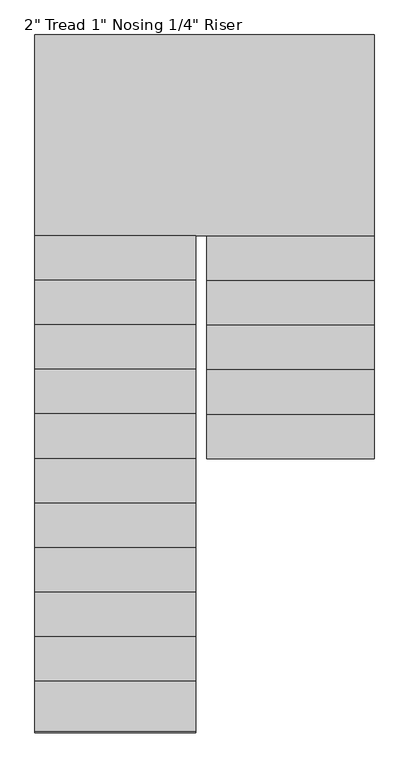
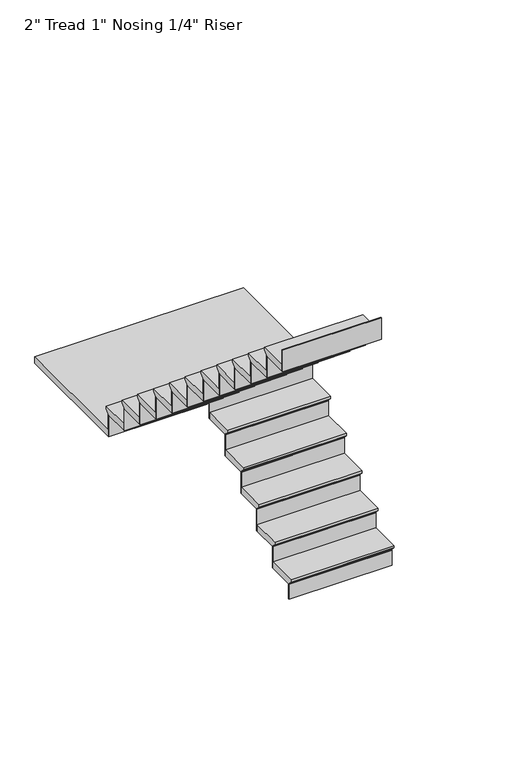
"""IFC4 building model written with IfcOpenShell, lengths in millimetres: stair flight geometry."""

from ifc_helpers import new_model, si_unit, origin, place, context, project, spatial, faceted_brep, source, transform, mapped, element, save


def stair_flight_16fb6ac5(model_context):
    return source(origin(), model_context, "Body", "Brep", [
        faceted_brep([(-3749.597125, 2714.6319226, 36573.8833333), (-3749.597125, 2714.6319226, 36592.9333333), (-4512.2136682, 2714.6319226, 36592.9333333), (-4512.2136682, 2714.6319226, 36573.8833333), (-3749.597125, 2740.0319226, 36548.4833333), (-4512.2136682, 2740.0319226, 36548.4833333), (-3749.597125, 2943.2319226, 36592.9333333), (-4512.2136682, 2943.2319226, 36592.9333333), (-4512.2136682, 2740.0319226, 36542.1333333), (-4512.2136682, 2943.2319226, 36542.1333333), (-3749.597125, 2943.2319226, 36542.1333333), (-3749.597125, 2740.0319226, 36542.1333333)], [[[0, 1, 2, 3]], [[4, 0, 3, 5]], [[2, 1, 6, 7]], [[8, 9, 10, 11]], [[2, 7, 9, 8, 5, 3]], [[8, 11, 4, 5]], [[6, 1, 0, 4, 11, 10]], [[7, 6, 10, 9]]]),
        faceted_brep([(-3749.597125, 2740.0319226, 36542.1333333), (-3749.597125, 2740.0319226, 36423.6), (-3749.597125, 2746.3819226, 36423.6), (-3749.597125, 2746.3819226, 36542.1333333), (-4512.2136682, 2740.0319226, 36542.1333333), (-4512.2136682, 2746.3819226, 36542.1333333), (-4512.2136682, 2746.3819226, 36423.6), (-4512.2136682, 2740.0319226, 36423.6)], [[[0, 1, 2, 3]], [[4, 5, 6, 7]], [[1, 0, 4, 7]], [[2, 1, 7, 6]], [[3, 2, 6, 5]], [[0, 3, 5, 4]]]),
        faceted_brep([(-3749.597125, 2943.2319226, 36711.4666667), (-3749.597125, 2943.2319226, 36542.1333333), (-3749.597125, 2949.5819226, 36542.1333333), (-3749.597125, 2949.5819226, 36711.4666667), (-4512.2136682, 2943.2319226, 36711.4666667), (-4512.2136682, 2949.5819226, 36711.4666667), (-4512.2136682, 2949.5819226, 36542.1333333), (-4512.2136682, 2943.2319226, 36542.1333333)], [[[0, 1, 2, 3]], [[4, 5, 6, 7]], [[1, 0, 4, 7]], [[2, 1, 7, 6]], [[3, 2, 6, 5]], [[0, 3, 5, 4]]]),
        faceted_brep([(-4512.2136682, 2917.8319226, 36762.2666667), (-3749.597125, 2917.8319226, 36762.2666667), (-3749.597125, 3146.4319226, 36762.2666667), (-4512.2136682, 3146.4319226, 36762.2666667), (-4512.2136682, 2943.2319226, 36711.4666667), (-4512.2136682, 3146.4319226, 36711.4666667), (-3749.597125, 3146.4319226, 36711.4666667), (-3749.597125, 2943.2319226, 36711.4666667), (-4512.2136682, 2943.2319226, 36717.8166667), (-4512.2136682, 2917.8319226, 36743.2166667), (-3749.597125, 2943.2319226, 36717.8166667), (-3749.597125, 2917.8319226, 36743.2166667)], [[[0, 1, 2, 3]], [[4, 5, 6, 7]], [[0, 3, 5, 4, 8, 9]], [[4, 7, 10, 8]], [[2, 1, 11, 10, 7, 6]], [[3, 2, 6, 5]], [[11, 1, 0, 9]], [[10, 11, 9, 8]]]),
        faceted_brep([(-3749.597125, 3146.4319226, 36880.8), (-3749.597125, 3146.4319226, 36711.4666667), (-3749.597125, 3152.7819226, 36711.4666667), (-3749.597125, 3152.7819226, 36880.8), (-4512.2136682, 3146.4319226, 36880.8), (-4512.2136682, 3152.7819226, 36880.8), (-4512.2136682, 3152.7819226, 36711.4666667), (-4512.2136682, 3146.4319226, 36711.4666667)], [[[0, 1, 2, 3]], [[4, 5, 6, 7]], [[1, 0, 4, 7]], [[2, 1, 7, 6]], [[3, 2, 6, 5]], [[0, 3, 5, 4]]]),
        faceted_brep([(-4512.2136682, 3121.0319226, 36931.6), (-3749.597125, 3121.0319226, 36931.6), (-3749.597125, 3349.6319226, 36931.6), (-4512.2136682, 3349.6319226, 36931.6), (-4512.2136682, 3146.4319226, 36880.8), (-4512.2136682, 3349.6319226, 36880.8), (-3749.597125, 3349.6319226, 36880.8), (-3749.597125, 3146.4319226, 36880.8), (-4512.2136682, 3146.4319226, 36887.15), (-4512.2136682, 3121.0319226, 36912.55), (-3749.597125, 3146.4319226, 36887.15), (-3749.597125, 3121.0319226, 36912.55)], [[[0, 1, 2, 3]], [[4, 5, 6, 7]], [[0, 3, 5, 4, 8, 9]], [[4, 7, 10, 8]], [[2, 1, 11, 10, 7, 6]], [[3, 2, 6, 5]], [[11, 1, 0, 9]], [[10, 11, 9, 8]]]),
        faceted_brep([(-3749.597125, 3349.6319226, 37050.1333333), (-3749.597125, 3349.6319226, 36880.8), (-3749.597125, 3355.9819226, 36880.8), (-3749.597125, 3355.9819226, 37050.1333333), (-4512.2136682, 3349.6319226, 37050.1333333), (-4512.2136682, 3355.9819226, 37050.1333333), (-4512.2136682, 3355.9819226, 36880.8), (-4512.2136682, 3349.6319226, 36880.8)], [[[0, 1, 2, 3]], [[4, 5, 6, 7]], [[1, 0, 4, 7]], [[2, 1, 7, 6]], [[3, 2, 6, 5]], [[0, 3, 5, 4]]]),
        faceted_brep([(-4512.2136682, 3324.2319226, 37100.9333333), (-3749.597125, 3324.2319226, 37100.9333333), (-3749.597125, 3552.8319226, 37100.9333333), (-4512.2136682, 3552.8319226, 37100.9333333), (-4512.2136682, 3349.6319226, 37050.1333333), (-4512.2136682, 3552.8319226, 37050.1333333), (-3749.597125, 3552.8319226, 37050.1333333), (-3749.597125, 3349.6319226, 37050.1333333), (-4512.2136682, 3349.6319226, 37056.4833333), (-4512.2136682, 3324.2319226, 37081.8833333), (-3749.597125, 3349.6319226, 37056.4833333), (-3749.597125, 3324.2319226, 37081.8833333)], [[[0, 1, 2, 3]], [[4, 5, 6, 7]], [[0, 3, 5, 4, 8, 9]], [[4, 7, 10, 8]], [[2, 1, 11, 10, 7, 6]], [[3, 2, 6, 5]], [[11, 1, 0, 9]], [[10, 11, 9, 8]]]),
        faceted_brep([(-3749.597125, 3552.8319226, 37219.4666667), (-3749.597125, 3552.8319226, 37050.1333333), (-3749.597125, 3559.1819226, 37050.1333333), (-3749.597125, 3559.1819226, 37219.4666667), (-4512.2136682, 3552.8319226, 37219.4666667), (-4512.2136682, 3559.1819226, 37219.4666667), (-4512.2136682, 3559.1819226, 37050.1333333), (-4512.2136682, 3552.8319226, 37050.1333333)], [[[0, 1, 2, 3]], [[4, 5, 6, 7]], [[1, 0, 4, 7]], [[2, 1, 7, 6]], [[3, 2, 6, 5]], [[0, 3, 5, 4]]]),
        faceted_brep([(-4512.2136682, 3527.4319226, 37270.2666667), (-3749.597125, 3527.4319226, 37270.2666667), (-3749.597125, 3756.0319226, 37270.2666667), (-4512.2136682, 3756.0319226, 37270.2666667), (-4512.2136682, 3552.8319226, 37219.4666667), (-4512.2136682, 3756.0319226, 37219.4666667), (-3749.597125, 3756.0319226, 37219.4666667), (-3749.597125, 3552.8319226, 37219.4666667), (-4512.2136682, 3552.8319226, 37225.8166667), (-4512.2136682, 3527.4319226, 37251.2166667), (-3749.597125, 3552.8319226, 37225.8166667), (-3749.597125, 3527.4319226, 37251.2166667)], [[[0, 1, 2, 3]], [[4, 5, 6, 7]], [[0, 3, 5, 4, 8, 9]], [[4, 7, 10, 8]], [[2, 1, 11, 10, 7, 6]], [[3, 2, 6, 5]], [[11, 1, 0, 9]], [[10, 11, 9, 8]]]),
        faceted_brep([(-3749.597125, 3756.0319226, 37388.8), (-3749.597125, 3756.0319226, 37219.4666667), (-3749.597125, 3762.3819226, 37219.4666667), (-3749.597125, 3762.3819226, 37388.8), (-4512.2136682, 3756.0319226, 37388.8), (-4512.2136682, 3762.3819226, 37388.8), (-4512.2136682, 3762.3819226, 37219.4666667), (-4512.2136682, 3756.0319226, 37219.4666667)], [[[0, 1, 2, 3]], [[4, 5, 6, 7]], [[1, 0, 4, 7]], [[2, 1, 7, 6]], [[3, 2, 6, 5]], [[0, 3, 5, 4]]]),
        faceted_brep([(-4563.0136682, 3705.2319226, 37439.6), (-4563.0136682, 3730.6319226, 37439.6), (-3749.597125, 3730.6319226, 37439.6), (-3749.597125, 4645.0319226, 37439.6), (-5295.0246464, 4645.0319226, 37439.6), (-5295.0246464, 3705.2319226, 37439.6), (-4563.0136682, 3730.6319226, 37388.8), (-4563.0136682, 3705.2319226, 37388.8), (-5295.0246464, 3705.2319226, 37388.8), (-5295.0246464, 4645.0319226, 37388.8), (-3749.597125, 4645.0319226, 37388.8), (-3749.597125, 3756.0319226, 37388.8), (-4512.2136682, 3756.0319226, 37388.8), (-4512.2136682, 3730.6319226, 37388.8), (-4512.2136682, 3730.6319226, 37420.55), (-3749.597125, 3730.6319226, 37420.55), (-4512.2136682, 3756.0319226, 37395.15), (-3749.597125, 3756.0319226, 37395.15)], [[[0, 1, 2, 3, 4, 5]], [[6, 7, 8, 9, 10, 11, 12, 13]], [[1, 0, 7, 6]], [[2, 1, 6, 13, 14, 15]], [[13, 12, 16, 14]], [[12, 11, 17, 16]], [[3, 2, 15, 17, 11, 10]], [[4, 3, 10, 9]], [[5, 4, 9, 8]], [[0, 5, 8, 7]], [[17, 15, 14, 16]]]),
        faceted_brep([(-5295.0246464, 3705.2319226, 37558.1333333), (-5295.0246464, 3705.2319226, 37388.8), (-5295.0246464, 3698.8819226, 37388.8), (-5295.0246464, 3698.8819226, 37558.1333333), (-4563.0136682, 3705.2319226, 37558.1333333), (-4563.0136682, 3698.8819226, 37558.1333333), (-4563.0136682, 3698.8819226, 37388.8), (-4563.0136682, 3705.2319226, 37388.8)], [[[0, 1, 2, 3]], [[4, 5, 6, 7]], [[1, 0, 4, 7]], [[2, 1, 7, 6]], [[3, 2, 6, 5]], [[0, 3, 5, 4]]]),
        faceted_brep([(-4563.0136682, 3730.6319226, 37608.9333333), (-5295.0246464, 3730.6319226, 37608.9333333), (-5295.0246464, 3502.0319226, 37608.9333333), (-4563.0136682, 3502.0319226, 37608.9333333), (-4563.0136682, 3705.2319226, 37558.1333333), (-4563.0136682, 3502.0319226, 37558.1333333), (-5295.0246464, 3502.0319226, 37558.1333333), (-5295.0246464, 3705.2319226, 37558.1333333), (-4563.0136682, 3705.2319226, 37564.4833333), (-4563.0136682, 3730.6319226, 37589.8833333), (-5295.0246464, 3705.2319226, 37564.4833333), (-5295.0246464, 3730.6319226, 37589.8833333)], [[[0, 1, 2, 3]], [[4, 5, 6, 7]], [[0, 3, 5, 4, 8, 9]], [[4, 7, 10, 8]], [[2, 1, 11, 10, 7, 6]], [[3, 2, 6, 5]], [[11, 1, 0, 9]], [[10, 11, 9, 8]]]),
        faceted_brep([(-5295.0246464, 3502.0319226, 37727.4666667), (-5295.0246464, 3502.0319226, 37558.1333333), (-5295.0246464, 3495.6819226, 37558.1333333), (-5295.0246464, 3495.6819226, 37727.4666667), (-4563.0136682, 3502.0319226, 37727.4666667), (-4563.0136682, 3495.6819226, 37727.4666667), (-4563.0136682, 3495.6819226, 37558.1333333), (-4563.0136682, 3502.0319226, 37558.1333333)], [[[0, 1, 2, 3]], [[4, 5, 6, 7]], [[1, 0, 4, 7]], [[2, 1, 7, 6]], [[3, 2, 6, 5]], [[0, 3, 5, 4]]]),
        faceted_brep([(-4563.0136682, 3527.4319226, 37778.2666667), (-5295.0246464, 3527.4319226, 37778.2666667), (-5295.0246464, 3298.8319226, 37778.2666667), (-4563.0136682, 3298.8319226, 37778.2666667), (-4563.0136682, 3502.0319226, 37727.4666667), (-4563.0136682, 3298.8319226, 37727.4666667), (-5295.0246464, 3298.8319226, 37727.4666667), (-5295.0246464, 3502.0319226, 37727.4666667), (-4563.0136682, 3502.0319226, 37733.8166667), (-4563.0136682, 3527.4319226, 37759.2166667), (-5295.0246464, 3502.0319226, 37733.8166667), (-5295.0246464, 3527.4319226, 37759.2166667)], [[[0, 1, 2, 3]], [[4, 5, 6, 7]], [[0, 3, 5, 4, 8, 9]], [[4, 7, 10, 8]], [[2, 1, 11, 10, 7, 6]], [[3, 2, 6, 5]], [[11, 1, 0, 9]], [[10, 11, 9, 8]]]),
        faceted_brep([(-5295.0246464, 3298.8319226, 37896.8), (-5295.0246464, 3298.8319226, 37727.4666667), (-5295.0246464, 3292.4819226, 37727.4666667), (-5295.0246464, 3292.4819226, 37896.8), (-4563.0136682, 3298.8319226, 37896.8), (-4563.0136682, 3292.4819226, 37896.8), (-4563.0136682, 3292.4819226, 37727.4666667), (-4563.0136682, 3298.8319226, 37727.4666667)], [[[0, 1, 2, 3]], [[4, 5, 6, 7]], [[1, 0, 4, 7]], [[2, 1, 7, 6]], [[3, 2, 6, 5]], [[0, 3, 5, 4]]]),
        faceted_brep([(-4563.0136682, 3324.2319226, 37947.6), (-5295.0246464, 3324.2319226, 37947.6), (-5295.0246464, 3095.6319226, 37947.6), (-4563.0136682, 3095.6319226, 37947.6), (-4563.0136682, 3298.8319226, 37896.8), (-4563.0136682, 3095.6319226, 37896.8), (-5295.0246464, 3095.6319226, 37896.8), (-5295.0246464, 3298.8319226, 37896.8), (-4563.0136682, 3298.8319226, 37903.15), (-4563.0136682, 3324.2319226, 37928.55), (-5295.0246464, 3298.8319226, 37903.15), (-5295.0246464, 3324.2319226, 37928.55)], [[[0, 1, 2, 3]], [[4, 5, 6, 7]], [[0, 3, 5, 4, 8, 9]], [[4, 7, 10, 8]], [[2, 1, 11, 10, 7, 6]], [[3, 2, 6, 5]], [[11, 1, 0, 9]], [[10, 11, 9, 8]]]),
        faceted_brep([(-5295.0246464, 3095.6319226, 38066.1333333), (-5295.0246464, 3095.6319226, 37896.8), (-5295.0246464, 3089.2819226, 37896.8), (-5295.0246464, 3089.2819226, 38066.1333333), (-4563.0136682, 3095.6319226, 38066.1333333), (-4563.0136682, 3089.2819226, 38066.1333333), (-4563.0136682, 3089.2819226, 37896.8), (-4563.0136682, 3095.6319226, 37896.8)], [[[0, 1, 2, 3]], [[4, 5, 6, 7]], [[1, 0, 4, 7]], [[2, 1, 7, 6]], [[3, 2, 6, 5]], [[0, 3, 5, 4]]]),
        faceted_brep([(-4563.0136682, 3121.0319226, 38116.9333333), (-5295.0246464, 3121.0319226, 38116.9333333), (-5295.0246464, 2892.4319226, 38116.9333333), (-4563.0136682, 2892.4319226, 38116.9333333), (-4563.0136682, 3095.6319226, 38066.1333333), (-4563.0136682, 2892.4319226, 38066.1333333), (-5295.0246464, 2892.4319226, 38066.1333333), (-5295.0246464, 3095.6319226, 38066.1333333), (-4563.0136682, 3095.6319226, 38072.4833333), (-4563.0136682, 3121.0319226, 38097.8833333), (-5295.0246464, 3095.6319226, 38072.4833333), (-5295.0246464, 3121.0319226, 38097.8833333)], [[[0, 1, 2, 3]], [[4, 5, 6, 7]], [[0, 3, 5, 4, 8, 9]], [[4, 7, 10, 8]], [[2, 1, 11, 10, 7, 6]], [[3, 2, 6, 5]], [[11, 1, 0, 9]], [[10, 11, 9, 8]]]),
        faceted_brep([(-5295.0246464, 2892.4319226, 38235.4666667), (-5295.0246464, 2892.4319226, 38066.1333333), (-5295.0246464, 2886.0819226, 38066.1333333), (-5295.0246464, 2886.0819226, 38235.4666667), (-4563.0136682, 2892.4319226, 38235.4666667), (-4563.0136682, 2886.0819226, 38235.4666667), (-4563.0136682, 2886.0819226, 38066.1333333), (-4563.0136682, 2892.4319226, 38066.1333333)], [[[0, 1, 2, 3]], [[4, 5, 6, 7]], [[1, 0, 4, 7]], [[2, 1, 7, 6]], [[3, 2, 6, 5]], [[0, 3, 5, 4]]]),
        faceted_brep([(-4563.0136682, 2917.8319226, 38286.2666667), (-5295.0246464, 2917.8319226, 38286.2666667), (-5295.0246464, 2689.2319226, 38286.2666667), (-4563.0136682, 2689.2319226, 38286.2666667), (-4563.0136682, 2892.4319226, 38235.4666667), (-4563.0136682, 2689.2319226, 38235.4666667), (-5295.0246464, 2689.2319226, 38235.4666667), (-5295.0246464, 2892.4319226, 38235.4666667), (-4563.0136682, 2892.4319226, 38241.8166667), (-4563.0136682, 2917.8319226, 38267.2166667), (-5295.0246464, 2892.4319226, 38241.8166667), (-5295.0246464, 2917.8319226, 38267.2166667)], [[[0, 1, 2, 3]], [[4, 5, 6, 7]], [[0, 3, 5, 4, 8, 9]], [[4, 7, 10, 8]], [[2, 1, 11, 10, 7, 6]], [[3, 2, 6, 5]], [[11, 1, 0, 9]], [[10, 11, 9, 8]]]),
        faceted_brep([(-5295.0246464, 2689.2319226, 38404.8), (-5295.0246464, 2689.2319226, 38235.4666667), (-5295.0246464, 2682.8819226, 38235.4666667), (-5295.0246464, 2682.8819226, 38404.8), (-4563.0136682, 2689.2319226, 38404.8), (-4563.0136682, 2682.8819226, 38404.8), (-4563.0136682, 2682.8819226, 38235.4666667), (-4563.0136682, 2689.2319226, 38235.4666667)], [[[0, 1, 2, 3]], [[4, 5, 6, 7]], [[1, 0, 4, 7]], [[2, 1, 7, 6]], [[3, 2, 6, 5]], [[0, 3, 5, 4]]]),
        faceted_brep([(-4563.0136682, 2714.6319226, 38455.6), (-5295.0246464, 2714.6319226, 38455.6), (-5295.0246464, 2486.0319226, 38455.6), (-4563.0136682, 2486.0319226, 38455.6), (-4563.0136682, 2689.2319226, 38404.8), (-4563.0136682, 2486.0319226, 38404.8), (-5295.0246464, 2486.0319226, 38404.8), (-5295.0246464, 2689.2319226, 38404.8), (-4563.0136682, 2689.2319226, 38411.15), (-4563.0136682, 2714.6319226, 38436.55), (-5295.0246464, 2689.2319226, 38411.15), (-5295.0246464, 2714.6319226, 38436.55)], [[[0, 1, 2, 3]], [[4, 5, 6, 7]], [[0, 3, 5, 4, 8, 9]], [[4, 7, 10, 8]], [[2, 1, 11, 10, 7, 6]], [[3, 2, 6, 5]], [[11, 1, 0, 9]], [[10, 11, 9, 8]]]),
        faceted_brep([(-5295.0246464, 2486.0319226, 38574.1333333), (-5295.0246464, 2486.0319226, 38404.8), (-5295.0246464, 2479.6819226, 38404.8), (-5295.0246464, 2479.6819226, 38574.1333333), (-4563.0136682, 2486.0319226, 38574.1333333), (-4563.0136682, 2479.6819226, 38574.1333333), (-4563.0136682, 2479.6819226, 38404.8), (-4563.0136682, 2486.0319226, 38404.8)], [[[0, 1, 2, 3]], [[4, 5, 6, 7]], [[1, 0, 4, 7]], [[2, 1, 7, 6]], [[3, 2, 6, 5]], [[0, 3, 5, 4]]]),
        faceted_brep([(-4563.0136682, 2511.4319226, 38624.9333333), (-5295.0246464, 2511.4319226, 38624.9333333), (-5295.0246464, 2282.8319226, 38624.9333333), (-4563.0136682, 2282.8319226, 38624.9333333), (-4563.0136682, 2486.0319226, 38574.1333333), (-4563.0136682, 2282.8319226, 38574.1333333), (-5295.0246464, 2282.8319226, 38574.1333333), (-5295.0246464, 2486.0319226, 38574.1333333), (-4563.0136682, 2486.0319226, 38580.4833333), (-4563.0136682, 2511.4319226, 38605.8833333), (-5295.0246464, 2486.0319226, 38580.4833333), (-5295.0246464, 2511.4319226, 38605.8833333)], [[[0, 1, 2, 3]], [[4, 5, 6, 7]], [[0, 3, 5, 4, 8, 9]], [[4, 7, 10, 8]], [[2, 1, 11, 10, 7, 6]], [[3, 2, 6, 5]], [[11, 1, 0, 9]], [[10, 11, 9, 8]]]),
        faceted_brep([(-5295.0246464, 2282.8319226, 38743.4666667), (-5295.0246464, 2282.8319226, 38574.1333333), (-5295.0246464, 2276.4819226, 38574.1333333), (-5295.0246464, 2276.4819226, 38743.4666667), (-4563.0136682, 2282.8319226, 38743.4666667), (-4563.0136682, 2276.4819226, 38743.4666667), (-4563.0136682, 2276.4819226, 38574.1333333), (-4563.0136682, 2282.8319226, 38574.1333333)], [[[0, 1, 2, 3]], [[4, 5, 6, 7]], [[1, 0, 4, 7]], [[2, 1, 7, 6]], [[3, 2, 6, 5]], [[0, 3, 5, 4]]]),
        faceted_brep([(-4563.0136682, 2308.2319226, 38794.2666667), (-5295.0246464, 2308.2319226, 38794.2666667), (-5295.0246464, 2079.6319226, 38794.2666667), (-4563.0136682, 2079.6319226, 38794.2666667), (-4563.0136682, 2282.8319226, 38743.4666667), (-4563.0136682, 2079.6319226, 38743.4666667), (-5295.0246464, 2079.6319226, 38743.4666667), (-5295.0246464, 2282.8319226, 38743.4666667), (-4563.0136682, 2282.8319226, 38749.8166667), (-4563.0136682, 2308.2319226, 38775.2166667), (-5295.0246464, 2282.8319226, 38749.8166667), (-5295.0246464, 2308.2319226, 38775.2166667)], [[[0, 1, 2, 3]], [[4, 5, 6, 7]], [[0, 3, 5, 4, 8, 9]], [[4, 7, 10, 8]], [[2, 1, 11, 10, 7, 6]], [[3, 2, 6, 5]], [[11, 1, 0, 9]], [[10, 11, 9, 8]]]),
        faceted_brep([(-5295.0246464, 2079.6319226, 38912.8), (-5295.0246464, 2079.6319226, 38743.4666667), (-5295.0246464, 2073.2819226, 38743.4666667), (-5295.0246464, 2073.2819226, 38912.8), (-4563.0136682, 2079.6319226, 38912.8), (-4563.0136682, 2073.2819226, 38912.8), (-4563.0136682, 2073.2819226, 38743.4666667), (-4563.0136682, 2079.6319226, 38743.4666667)], [[[0, 1, 2, 3]], [[4, 5, 6, 7]], [[1, 0, 4, 7]], [[2, 1, 7, 6]], [[3, 2, 6, 5]], [[0, 3, 5, 4]]]),
        faceted_brep([(-4563.0136682, 2105.0319226, 38963.6), (-5295.0246464, 2105.0319226, 38963.6), (-5295.0246464, 1876.4319226, 38963.6), (-4563.0136682, 1876.4319226, 38963.6), (-4563.0136682, 2079.6319226, 38912.8), (-4563.0136682, 1876.4319226, 38912.8), (-5295.0246464, 1876.4319226, 38912.8), (-5295.0246464, 2079.6319226, 38912.8), (-4563.0136682, 2079.6319226, 38919.15), (-4563.0136682, 2105.0319226, 38944.55), (-5295.0246464, 2079.6319226, 38919.15), (-5295.0246464, 2105.0319226, 38944.55)], [[[0, 1, 2, 3]], [[4, 5, 6, 7]], [[0, 3, 5, 4, 8, 9]], [[4, 7, 10, 8]], [[2, 1, 11, 10, 7, 6]], [[3, 2, 6, 5]], [[11, 1, 0, 9]], [[10, 11, 9, 8]]]),
        faceted_brep([(-5295.0246464, 1876.4319226, 39082.1333333), (-5295.0246464, 1876.4319226, 38912.8), (-5295.0246464, 1870.0819226, 38912.8), (-5295.0246464, 1870.0819226, 39082.1333333), (-4563.0136682, 1876.4319226, 39082.1333333), (-4563.0136682, 1870.0819226, 39082.1333333), (-4563.0136682, 1870.0819226, 38912.8), (-4563.0136682, 1876.4319226, 38912.8)], [[[0, 1, 2, 3]], [[4, 5, 6, 7]], [[1, 0, 4, 7]], [[2, 1, 7, 6]], [[3, 2, 6, 5]], [[0, 3, 5, 4]]]),
        faceted_brep([(-4563.0136682, 1901.8319226, 39132.9333333), (-5295.0246464, 1901.8319226, 39132.9333333), (-5295.0246464, 1673.2319226, 39132.9333333), (-4563.0136682, 1673.2319226, 39132.9333333), (-4563.0136682, 1876.4319226, 39082.1333333), (-4563.0136682, 1673.2319226, 39082.1333333), (-5295.0246464, 1673.2319226, 39082.1333333), (-5295.0246464, 1876.4319226, 39082.1333333), (-4563.0136682, 1876.4319226, 39088.4833333), (-4563.0136682, 1901.8319226, 39113.8833333), (-5295.0246464, 1876.4319226, 39088.4833333), (-5295.0246464, 1901.8319226, 39113.8833333)], [[[0, 1, 2, 3]], [[4, 5, 6, 7]], [[0, 3, 5, 4, 8, 9]], [[4, 7, 10, 8]], [[2, 1, 11, 10, 7, 6]], [[3, 2, 6, 5]], [[11, 1, 0, 9]], [[10, 11, 9, 8]]]),
        faceted_brep([(-5295.0246464, 1673.2319226, 39251.4666667), (-5295.0246464, 1673.2319226, 39082.1333333), (-5295.0246464, 1666.8819226, 39082.1333333), (-5295.0246464, 1666.8819226, 39251.4666667), (-4563.0136682, 1673.2319226, 39251.4666667), (-4563.0136682, 1666.8819226, 39251.4666667), (-4563.0136682, 1666.8819226, 39082.1333333), (-4563.0136682, 1673.2319226, 39082.1333333)], [[[0, 1, 2, 3]], [[4, 5, 6, 7]], [[1, 0, 4, 7]], [[2, 1, 7, 6]], [[3, 2, 6, 5]], [[0, 3, 5, 4]]]),
        faceted_brep([(-4563.0136682, 1698.6319226, 39302.2666667), (-5295.0246464, 1698.6319226, 39302.2666667), (-5295.0246464, 1470.0319226, 39302.2666667), (-4563.0136682, 1470.0319226, 39302.2666667), (-4563.0136682, 1673.2319226, 39251.4666667), (-4563.0136682, 1470.0319226, 39251.4666667), (-5295.0246464, 1470.0319226, 39251.4666667), (-5295.0246464, 1673.2319226, 39251.4666667), (-4563.0136682, 1673.2319226, 39257.8166667), (-4563.0136682, 1698.6319226, 39283.2166667), (-5295.0246464, 1673.2319226, 39257.8166667), (-5295.0246464, 1698.6319226, 39283.2166667)], [[[0, 1, 2, 3]], [[4, 5, 6, 7]], [[0, 3, 5, 4, 8, 9]], [[4, 7, 10, 8]], [[2, 1, 11, 10, 7, 6]], [[3, 2, 6, 5]], [[11, 1, 0, 9]], [[10, 11, 9, 8]]]),
        faceted_brep([(-5295.0246464, 1470.0319226, 39420.8), (-5295.0246464, 1470.0319226, 39251.4666667), (-5295.0246464, 1463.6819226, 39251.4666667), (-5295.0246464, 1463.6819226, 39420.8), (-4563.0136682, 1470.0319226, 39420.8), (-4563.0136682, 1463.6819226, 39420.8), (-4563.0136682, 1463.6819226, 39251.4666667), (-4563.0136682, 1470.0319226, 39251.4666667)], [[[0, 1, 2, 3]], [[4, 5, 6, 7]], [[1, 0, 4, 7]], [[2, 1, 7, 6]], [[3, 2, 6, 5]], [[0, 3, 5, 4]]]),
    ])


if __name__ == "__main__":
    model = new_model("IFC4")
    model_context = context("Model", 3, world=origin())
    ifc_project = project(units=[si_unit("LENGTHUNIT", "METRE", prefix="MILLI")], contexts=[model_context])
    site = spatial("IfcSite", under=ifc_project)
    building = spatial("IfcBuilding", under=site)
    placement = place(None, origin())
    stair_flight_shape = stair_flight_16fb6ac5(model_context)
    element("IfcStairFlight", 1, ObjectType="2\" Tread 1\" Nosing 1/4\" Riser", at=placement, inside=building, context=model_context, shape_type="MappedRepresentation", body=[
        mapped(stair_flight_shape, transform((0.0, 0.0, 0.0), x_axis=(1.0, 0.0, 0.0), y_axis=(0.0, 1.0, 0.0), z_axis=(0.0, 0.0, 1.0))),
    ])
    save(model, "model.ifc")
